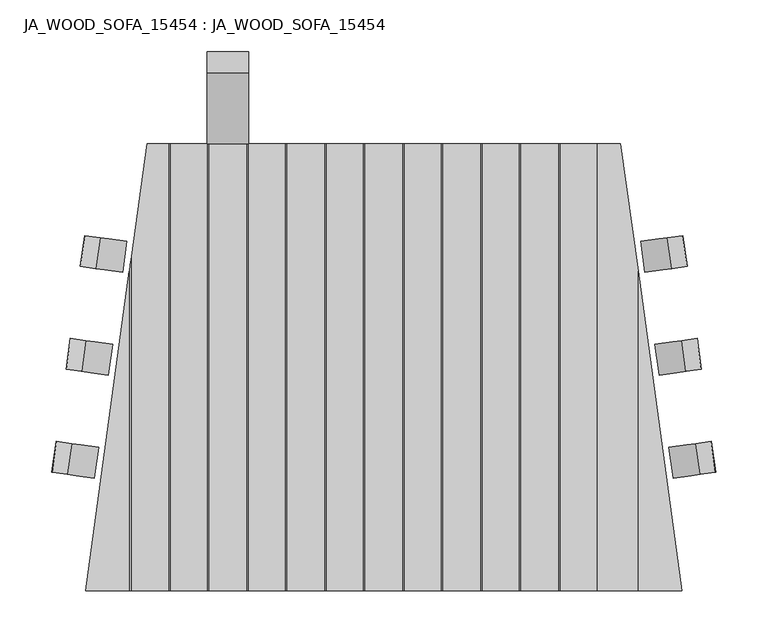
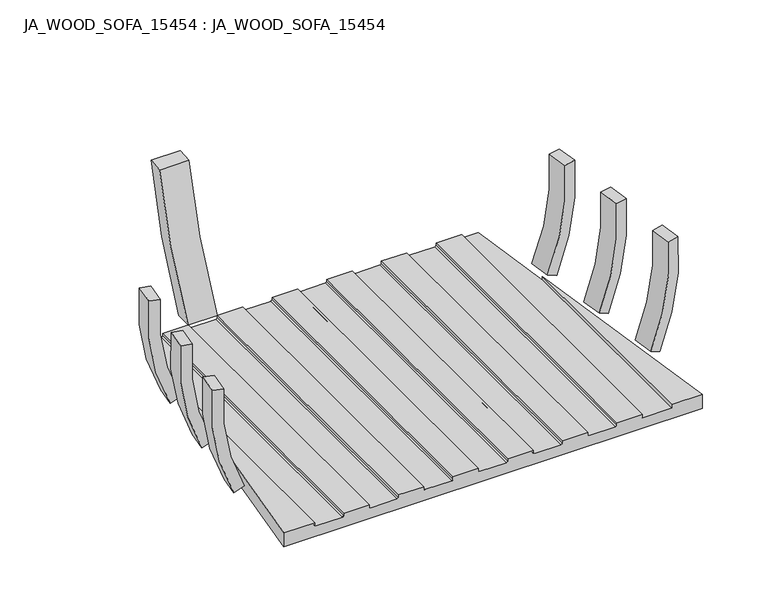
"""IFC4 building model written with IfcOpenShell, lengths in millimetres: furniture geometry, JA_WOOD_SOFA_15454 : JA_WOOD_SOFA_15454."""

from ifc_helpers import new_model, si_unit, point, frame, frame_2d, origin, origin_2d, place, context, project, spatial, polyline, circle_curve, ellipse_curve, trimmed, segment, composite_curve, outline, extrude, source, transform, mapped, element, save
from ifc_brep_helpers import plane_surface, revolved_surface, advanced_brep


def ja_wood_sofa_15454_ja_wood_sofa_15454_1d85e86b(model_context):
    return source(origin(), model_context, "Body", "SolidModel", [
        extrude(outline(composite_curve([segment(trimmed(circle_curve(frame_2d((-81.7276373, 616.3111076)), 600.0), [point((440.0, 320.0))], [point((507.7138581, 504.2453967))], True, "CARTESIAN"), True, "CONTINUOUS"), segment(polyline([(507.7138581, 504.2453967), (528.3899255, 506.0543182)]), True, "CONTINUOUS"), segment(trimmed(circle_curve(frame_2d((-81.7276373, 616.3111076)), 620.0), [point((528.3899255, 506.0543182))], [point((462.8820647, 320.0))], False, "CARTESIAN"), True, "CONTINUOUS"), segment(polyline([(462.8820647, 320.0), (440.0, 320.0)]), True, "CONTINUOUS")], self_intersect=False)), frame((-170.0, 0.0, 0.0), z_axis=(1.0, 0.0, 0.0), x_axis=(0.0, 1.0, 0.0)), (0.0, 0.0, 1.0), 40.0),
        extrude(outline(composite_curve([segment(trimmed(circle_curve(origin_2d(), 286.25), [point((246.9486899, -144.7598254))], [point((286.25, 0.0))], True, "CARTESIAN"), True, "CONTINUOUS"), segment(polyline([(286.25, 0.0), (301.2499999, -1e-07)]), True, "CONTINUOUS"), segment(trimmed(circle_curve(origin_2d(), 301.25), [point((301.2499999, -1e-07))], [point((259.8892326, -152.3454931))], False, "CARTESIAN"), True, "CONTINUOUS"), segment(polyline([(259.8892326, -152.3454931), (246.9486899, -144.7598254)]), True, "CONTINUOUS")], self_intersect=False)), frame((-22.2448942, 82.953428, 441.8308906), z_axis=(0.13632983976605592, 0.99066350230003, 0.0), x_axis=(-0.9866030973847555, 0.1357710684474402, 0.09044636644690265)), (0.0, 0.0, 1.0), 30.0),
        extrude(outline(composite_curve([segment(trimmed(circle_curve(origin_2d(), 286.25), [point((246.9486899, -144.7598254))], [point((286.25, 0.0))], True, "CARTESIAN"), True, "CONTINUOUS"), segment(polyline([(286.25, 0.0), (301.25, -1e-07)]), True, "CONTINUOUS"), segment(trimmed(circle_curve(origin_2d(), 301.25), [point((301.25, -1e-07))], [point((259.8892326, -152.3454931))], False, "CARTESIAN"), True, "CONTINUOUS"), segment(polyline([(259.8892326, -152.3454931), (246.9486899, -144.7598254)]), True, "CONTINUOUS")], self_intersect=False)), frame((-8.6188139, 182.0207281, 441.8308906), z_axis=(0.13632983976605592, 0.99066350230003, 0.0), x_axis=(-0.9866030973847555, 0.1357710684474402, 0.09044636644690265)), (0.0, 0.0, 1.0), 30.0),
        extrude(outline(composite_curve([segment(trimmed(circle_curve(origin_2d(), 286.25), [point((246.94869, -144.7598254))], [point((286.25, 0.0))], True, "CARTESIAN"), True, "CONTINUOUS"), segment(polyline([(286.25, 0.0), (301.25, -1e-07)]), True, "CONTINUOUS"), segment(trimmed(circle_curve(origin_2d(), 301.25), [point((301.25, -1e-07))], [point((259.8892326, -152.3454931))], False, "CARTESIAN"), True, "CONTINUOUS"), segment(polyline([(259.8892326, -152.3454931), (246.94869, -144.7598254)]), True, "CONTINUOUS")], self_intersect=False)), frame((5.0141701, 281.0870783, 441.8308906), z_axis=(0.13632983976605592, 0.99066350230003, 0.0), x_axis=(-0.9866030973847555, 0.1357710684474402, 0.09044636644690265)), (0.0, 0.0, 1.0), 30.0),
        extrude(outline(composite_curve([segment(trimmed(circle_curve(origin_2d(), 301.25), [point((259.8892326, 152.3454931))], [point((301.2499999, 1e-07))], False, "CARTESIAN"), True, "CONTINUOUS"), segment(polyline([(301.2499999, 1e-07), (286.25, 0.0)]), True, "CONTINUOUS"), segment(trimmed(circle_curve(origin_2d(), 286.25), [point((286.25, 0.0))], [point((246.9486899, 144.7598254))], True, "CARTESIAN"), True, "CONTINUOUS"), segment(polyline([(246.9486899, 144.7598254), (259.8892326, 152.3454931)]), True, "CONTINUOUS")], self_intersect=False)), frame((22.2448942, 82.953428, 441.8308906), z_axis=(-0.13632983976605592, 0.99066350230003, 0.0), x_axis=(0.9866030973847555, 0.1357710684474402, 0.09044636644690265)), (0.0, 0.0, 1.0), 30.0),
        extrude(outline(composite_curve([segment(trimmed(circle_curve(origin_2d(), 301.25), [point((259.8892326, 152.3454931))], [point((301.25, 1e-07))], False, "CARTESIAN"), True, "CONTINUOUS"), segment(polyline([(301.25, 1e-07), (286.25, 0.0)]), True, "CONTINUOUS"), segment(trimmed(circle_curve(origin_2d(), 286.25), [point((286.25, 0.0))], [point((246.9486899, 144.7598254))], True, "CARTESIAN"), True, "CONTINUOUS"), segment(polyline([(246.9486899, 144.7598254), (259.8892326, 152.3454931)]), True, "CONTINUOUS")], self_intersect=False)), frame((8.6188139, 182.0207281, 441.8308906), z_axis=(-0.13632983976605592, 0.99066350230003, 0.0), x_axis=(0.9866030973847555, 0.1357710684474402, 0.09044636644690265)), (0.0, 0.0, 1.0), 30.0),
        extrude(outline(composite_curve([segment(trimmed(circle_curve(origin_2d(), 301.25), [point((259.8892326, 152.3454931))], [point((301.25, 1e-07))], False, "CARTESIAN"), True, "CONTINUOUS"), segment(polyline([(301.25, 1e-07), (286.25, 0.0)]), True, "CONTINUOUS"), segment(trimmed(circle_curve(origin_2d(), 286.25), [point((286.25, 0.0))], [point((246.94869, 144.7598254))], True, "CARTESIAN"), True, "CONTINUOUS"), segment(polyline([(246.94869, 144.7598254), (259.8892326, 152.3454931)]), True, "CONTINUOUS")], self_intersect=False)), frame((-5.0141701, 281.0870783, 441.8308906), z_axis=(-0.13632983976605592, 0.99066350230003, 0.0), x_axis=(0.9866030973847555, 0.1357710684474402, 0.09044636644690265)), (0.0, 0.0, 1.0), 30.0),
        advanced_brep(
        [(-20.0, 10.0, 317.0), (-20.0, 440.0, 317.0), (-20.0, 440.0, 320.0), (-20.0, 10.0, 320.0), (18.0, 10.0, 315.0), (18.0, 440.0, 315.0), (-18.0, 440.0, 315.0), (-18.0, 10.0, 315.0), (20.0, 440.0, 317.0), (20.0, 10.0, 317.0), (20.0, 10.0, 320.0), (20.0, 440.0, 320.0), (55.0, 10.0, 317.0), (55.0, 440.0, 317.0), (55.0, 440.0, 320.0), (55.0, 10.0, 320.0), (93.0, 10.0, 315.0), (93.0, 440.0, 315.0), (57.0, 440.0, 315.0), (57.0, 10.0, 315.0), (95.0, 440.0, 317.0), (95.0, 10.0, 317.0), (95.0, 10.0, 320.0), (95.0, 440.0, 320.0), (130.0, 10.0, 317.0), (130.0, 440.0, 317.0), (130.0, 440.0, 320.0), (130.0, 10.0, 320.0), (168.0, 10.0, 315.0), (168.0, 440.0, 315.0), (132.0, 440.0, 315.0), (132.0, 10.0, 315.0), (170.0, 440.0, 317.0), (170.0, 10.0, 317.0), (170.0, 10.0, 320.0), (170.0, 440.0, 320.0), (-170.0, 10.0, 317.0), (-170.0, 440.0, 317.0), (-170.0, 440.0, 320.0), (-170.0, 10.0, 320.0), (-132.0, 10.0, 315.0), (-132.0, 440.0, 315.0), (-168.0, 440.0, 315.0), (-168.0, 10.0, 315.0), (-130.0, 440.0, 317.0), (-130.0, 10.0, 317.0), (-130.0, 10.0, 320.0), (-130.0, 440.0, 320.0), (-95.0, 10.0, 317.0), (-95.0, 440.0, 317.0), (-95.0, 440.0, 320.0), (-95.0, 10.0, 320.0), (-57.0, 10.0, 315.0), (-57.0, 440.0, 315.0), (-93.0, 440.0, 315.0), (-93.0, 10.0, 315.0), (-55.0, 440.0, 317.0), (-55.0, 10.0, 317.0), (-55.0, 10.0, 320.0), (-55.0, 440.0, 320.0), (-245.0, 10.0, 317.0), (-245.0, 317.1484871, 317.0), (-245.0, 317.1484871, 320.0), (-245.0, 10.0, 320.0), (-207.0, 10.0, 315.0), (-207.0, 440.0, 315.0), (-228.0938285, 440.0, 315.0), (-243.0, 331.6818204, 315.0), (-243.0, 10.0, 315.0), (-205.0, 440.0, 317.0), (-205.0, 10.0, 317.0), (-205.0, 10.0, 320.0), (-205.0, 440.0, 320.0), (205.0, 10.0, 315.0), (205.0, 440.0, 315.0), (205.0, 440.0, 320.0), (205.0, 10.0, 320.0), (245.0, 10.0, 315.0), (245.0, 317.1484871, 315.0), (228.0938285, 440.0, 315.0), (245.0, 10.0, 320.0), (245.0, 317.1484871, 320.0), (-287.2681404, 10.0, 320.0), (287.2681404, 10.0, 320.0), (-228.0938285, 440.0, 300.0), (228.0938285, 440.0, 300.0), (287.2681404, 10.0, 300.0), (-287.2681404, 10.0, 300.0)],
        [
            (0, 1),
            (1, 2),
            (2, 3),
            (3, 0),
            (4, 5),
            (5, 6),
            (6, 7),
            (7, 4),
            (8, 9),
            (9, 10),
            (10, 11),
            (11, 8),
            (12, 13),
            (13, 14),
            (14, 15),
            (15, 12),
            (16, 17),
            (17, 18),
            (18, 19),
            (19, 16),
            (20, 21),
            (21, 22),
            (22, 23),
            (23, 20),
            (24, 25),
            (25, 26),
            (26, 27),
            (27, 24),
            (28, 29),
            (29, 30),
            (30, 31),
            (31, 28),
            (32, 33),
            (33, 34),
            (34, 35),
            (35, 32),
            (36, 37),
            (37, 38),
            (38, 39),
            (39, 36),
            (40, 41),
            (41, 42),
            (42, 43),
            (43, 40),
            (44, 45),
            (45, 46),
            (46, 47),
            (47, 44),
            (48, 49),
            (49, 50),
            (50, 51),
            (51, 48),
            (52, 53),
            (53, 54),
            (54, 55),
            (55, 52),
            (56, 57),
            (57, 58),
            (58, 59),
            (59, 56),
            (60, 61),
            (61, 62),
            (62, 63),
            (63, 60),
            (64, 65),
            (65, 66),
            (66, 67),
            (67, 68),
            (68, 64),
            (69, 70),
            (70, 71),
            (71, 72),
            (72, 69),
            (73, 74),
            (74, 75),
            (75, 76),
            (76, 73),
            (73, 77),
            (77, 78),
            (78, 79),
            (79, 74),
            (77, 80),
            (80, 81),
            (81, 78),
            (62, 82),
            (82, 63),
            (10, 15),
            (14, 11),
            (22, 27),
            (26, 23),
            (46, 51),
            (50, 47),
            (58, 3),
            (2, 59),
            (71, 39),
            (38, 72),
            (34, 76),
            (75, 35),
            (80, 83),
            (83, 81),
            (84, 85),
            (85, 86),
            (86, 87),
            (87, 84),
            (87, 82),
            (61, 67, ellipse_curve(frame((-243.0, 331.6818204, 317.0), z_axis=(0.9906635023000295, -0.13632983976605914, 0.0), x_axis=(-0.13632983976605917, -0.9906635023000296, 0.0)), 14.6703026, 2.0)),
            (66, 84),
            (86, 83),
            (33, 28, circle_curve(frame((168.0, 10.0, 317.0), z_axis=(0.0, 1.0, 0.0), x_axis=(1.0, 0.0, 0.0)), 2.0)),
            (31, 24, circle_curve(frame((132.0, 10.0, 317.0), z_axis=(0.0, 1.0, 0.0), x_axis=(1.0, 0.0, 0.0)), 2.0)),
            (21, 16, circle_curve(frame((93.0, 10.0, 317.0), z_axis=(0.0, 1.0, 0.0), x_axis=(1.0, 0.0, 0.0)), 2.0)),
            (19, 12, circle_curve(frame((57.0, 10.0, 317.0), z_axis=(0.0, 1.0, 0.0), x_axis=(1.0, 0.0, 0.0)), 2.0)),
            (9, 4, circle_curve(frame((18.0, 10.0, 317.0), z_axis=(0.0, 1.0, 0.0), x_axis=(1.0, 0.0, 0.0)), 2.0)),
            (7, 0, circle_curve(frame((-18.0, 10.0, 317.0), z_axis=(0.0, 1.0, 0.0), x_axis=(1.0, 0.0, 0.0)), 2.0)),
            (57, 52, circle_curve(frame((-57.0, 10.0, 317.0), z_axis=(0.0, 1.0, 0.0), x_axis=(1.0, 0.0, 0.0)), 2.0)),
            (55, 48, circle_curve(frame((-93.0, 10.0, 317.0), z_axis=(0.0, 1.0, 0.0), x_axis=(1.0, 0.0, 0.0)), 2.0)),
            (45, 40, circle_curve(frame((-132.0, 10.0, 317.0), z_axis=(0.0, 1.0, 0.0), x_axis=(1.0, 0.0, 0.0)), 2.0)),
            (43, 36, circle_curve(frame((-168.0, 10.0, 317.0), z_axis=(0.0, 1.0, 0.0), x_axis=(1.0, 0.0, 0.0)), 2.0)),
            (70, 64, circle_curve(frame((-207.0, 10.0, 317.0), z_axis=(0.0, 1.0, 0.0), x_axis=(1.0, 0.0, 0.0)), 2.0)),
            (68, 60, circle_curve(frame((-243.0, 10.0, 317.0), z_axis=(0.0, 1.0, 0.0), x_axis=(1.0, 0.0, 0.0)), 2.0)),
            (85, 79),
            (65, 69, circle_curve(frame((-207.0, 440.0, 317.0), z_axis=(0.0, -1.0, 0.0), x_axis=(1.0, 0.0, 0.0)), 2.0)),
            (37, 42, circle_curve(frame((-168.0, 440.0, 317.0), z_axis=(0.0, -1.0, 0.0), x_axis=(1.0, 0.0, 0.0)), 2.0)),
            (41, 44, circle_curve(frame((-132.0, 440.0, 317.0), z_axis=(0.0, -1.0, 0.0), x_axis=(1.0, 0.0, 0.0)), 2.0)),
            (49, 54, circle_curve(frame((-93.0, 440.0, 317.0), z_axis=(0.0, -1.0, 0.0), x_axis=(1.0, 0.0, 0.0)), 2.0)),
            (53, 56, circle_curve(frame((-57.0, 440.0, 317.0), z_axis=(0.0, -1.0, 0.0), x_axis=(1.0, 0.0, 0.0)), 2.0)),
            (1, 6, circle_curve(frame((-18.0, 440.0, 317.0), z_axis=(0.0, -1.0, 0.0), x_axis=(1.0, 0.0, 0.0)), 2.0)),
            (5, 8, circle_curve(frame((18.0, 440.0, 317.0), z_axis=(0.0, -1.0, 0.0), x_axis=(1.0, 0.0, 0.0)), 2.0)),
            (13, 18, circle_curve(frame((57.0, 440.0, 317.0), z_axis=(0.0, -1.0, 0.0), x_axis=(1.0, 0.0, 0.0)), 2.0)),
            (17, 20, circle_curve(frame((93.0, 440.0, 317.0), z_axis=(0.0, -1.0, 0.0), x_axis=(1.0, 0.0, 0.0)), 2.0)),
            (25, 30, circle_curve(frame((132.0, 440.0, 317.0), z_axis=(0.0, -1.0, 0.0), x_axis=(1.0, 0.0, 0.0)), 2.0)),
            (29, 32, circle_curve(frame((168.0, 440.0, 317.0), z_axis=(0.0, -1.0, 0.0), x_axis=(1.0, 0.0, 0.0)), 2.0)),
        ],
        [
            plane_surface(frame((-20.0, 10.0, 320.0), z_axis=(1.0, 0.0, 0.0), x_axis=(0.0, 1.0, 0.0))),
            plane_surface(frame((-18.0, 10.0, 315.0), z_axis=(0.0, 0.0, 1.0), x_axis=(0.0, 1.0, 0.0))),
            plane_surface(frame((20.0, 10.0, 317.0), z_axis=(-1.0, 0.0, 0.0), x_axis=(0.0, 1.0, 0.0))),
            plane_surface(frame((55.0, 10.0, 320.0), z_axis=(1.0, 0.0, 0.0), x_axis=(0.0, 1.0, 0.0))),
            plane_surface(frame((57.0, 10.0, 315.0), z_axis=(0.0, 0.0, 1.0), x_axis=(0.0, 1.0, 0.0))),
            plane_surface(frame((95.0, 10.0, 317.0), z_axis=(-1.0, 0.0, 0.0), x_axis=(0.0, 1.0, 0.0))),
            plane_surface(frame((130.0, 10.0, 320.0), z_axis=(1.0, 0.0, 0.0), x_axis=(0.0, 1.0, 0.0))),
            plane_surface(frame((132.0, 10.0, 315.0), z_axis=(0.0, 0.0, 1.0), x_axis=(0.0, 1.0, 0.0))),
            plane_surface(frame((170.0, 10.0, 317.0), z_axis=(-1.0, 0.0, 0.0), x_axis=(0.0, 1.0, 0.0))),
            plane_surface(frame((-170.0, 10.0, 320.0), z_axis=(1.0, 0.0, 0.0), x_axis=(0.0, 1.0, 0.0))),
            plane_surface(frame((-168.0, 10.0, 315.0), z_axis=(0.0, 0.0, 1.0), x_axis=(0.0, 1.0, 0.0))),
            plane_surface(frame((-130.0, 10.0, 317.0), z_axis=(-1.0, 0.0, 0.0), x_axis=(0.0, 1.0, 0.0))),
            plane_surface(frame((-95.0, 10.0, 320.0), z_axis=(1.0, 0.0, 0.0), x_axis=(0.0, 1.0, 0.0))),
            plane_surface(frame((-93.0, 10.0, 315.0), z_axis=(0.0, 0.0, 1.0), x_axis=(0.0, 1.0, 0.0))),
            plane_surface(frame((-55.0, 10.0, 317.0), z_axis=(-1.0, 0.0, 0.0), x_axis=(0.0, 1.0, 0.0))),
            plane_surface(frame((-245.0, 10.0, 320.0), z_axis=(1.0, 0.0, 0.0), x_axis=(0.0, 1.0, 0.0))),
            plane_surface(frame((-243.0, 10.0, 315.0), z_axis=(0.0, 0.0, 1.0), x_axis=(0.0, 1.0, 0.0))),
            plane_surface(frame((-205.0, 10.0, 317.0), z_axis=(-1.0, 0.0, 0.0), x_axis=(0.0, 1.0, 0.0))),
            plane_surface(frame((205.0, 10.0, 320.0), z_axis=(1.0, 0.0, 0.0), x_axis=(0.0, 1.0, 0.0))),
            plane_surface(frame((205.0, 10.0, 315.0), z_axis=(0.0, 0.0, 1.0), x_axis=(0.0, 1.0, 0.0))),
            plane_surface(frame((245.0, 10.0, 315.0), z_axis=(-1.0, 0.0, 0.0), x_axis=(0.0, 1.0, 0.0))),
            plane_surface(frame((-287.6258394, 7.4007211, 320.0), z_axis=(0.0, 0.0, 1.0), x_axis=(-0.13632983976605914, -0.9906635023000295, 0.0))),
            plane_surface(frame((-287.6258394, 7.4007211, 300.0), z_axis=(0.0, 0.0, -1.0), x_axis=(0.13632983976605914, 0.9906635023000295, 0.0))),
            plane_surface(frame((-228.0938285, 440.0, 320.0), z_axis=(-0.9906635023000295, 0.13632983976605914, 0.0), x_axis=(0.0, 0.0, -1.0))),
            plane_surface(frame((-287.2681404, 10.0, 320.0), z_axis=(0.0, -1.0, 0.0), x_axis=(0.0, 0.0, -1.0))),
            plane_surface(frame((287.2681404, 10.0, 320.0), z_axis=(0.9906635023000295, 0.13632983976605914, 0.0), x_axis=(0.0, 0.0, -1.0))),
            plane_surface(frame((228.0938285, 440.0, 320.0), z_axis=(0.0, 1.0, 0.0), x_axis=(0.0, 0.0, -1.0))),
            revolved_surface(polyline([(-16.0, 10.0, 317.0), (-16.0, 440.0, 317.0)]), (-18.0, 440.0, 317.0), (0.0, -1.0, 0.0)),
            revolved_surface(polyline([(20.0, 10.0, 317.0), (20.0, 440.0, 317.0)]), (18.0, 440.0, 317.0), (0.0, -1.0, 0.0)),
            revolved_surface(polyline([(59.0, 10.0, 317.0), (59.0, 440.0, 317.0)]), (57.0, 440.0, 317.0), (0.0, -1.0, 0.0)),
            revolved_surface(polyline([(95.0, 10.0, 317.0), (95.0, 440.0, 317.0)]), (93.0, 440.0, 317.0), (0.0, -1.0, 0.0)),
            revolved_surface(polyline([(134.0, 10.0, 317.0), (134.0, 440.0, 317.0)]), (132.0, 440.0, 317.0), (0.0, -1.0, 0.0)),
            revolved_surface(polyline([(170.0, 10.0, 317.0), (170.0, 440.0, 317.0)]), (168.0, 440.0, 317.0), (0.0, -1.0, 0.0)),
            revolved_surface(polyline([(-166.0, 10.0, 317.0), (-166.0, 440.0, 317.0)]), (-168.0, 440.0, 317.0), (0.0, -1.0, 0.0)),
            revolved_surface(polyline([(-130.0, 10.0, 317.0), (-130.0, 440.0, 317.0)]), (-132.0, 440.0, 317.0), (0.0, -1.0, 0.0)),
            revolved_surface(polyline([(-91.0, 10.0, 317.0), (-91.0, 440.0, 317.0)]), (-93.0, 440.0, 317.0), (0.0, -1.0, 0.0)),
            revolved_surface(polyline([(-55.0, 10.0, 317.0), (-55.0, 440.0, 317.0)]), (-57.0, 440.0, 317.0), (0.0, -1.0, 0.0)),
            revolved_surface(polyline([(-241.0, 10.0, 317.0), (-241.0, 346.21515375351726, 317.0)]), (-243.0, 440.0, 317.0), (0.0, -1.0, 0.0)),
            revolved_surface(polyline([(-205.0, 10.0, 317.0), (-205.0, 440.0, 317.0)]), (-207.0, 440.0, 317.0), (0.0, -1.0, 0.0)),
        ],
        [
            (0, [[1, 2, 3, 4]]),
            (1, [[5, 6, 7, 8]]),
            (2, [[9, 10, 11, 12]]),
            (3, [[13, 14, 15, 16]]),
            (4, [[17, 18, 19, 20]]),
            (5, [[21, 22, 23, 24]]),
            (6, [[25, 26, 27, 28]]),
            (7, [[29, 30, 31, 32]]),
            (8, [[33, 34, 35, 36]]),
            (9, [[37, 38, 39, 40]]),
            (10, [[41, 42, 43, 44]]),
            (11, [[45, 46, 47, 48]]),
            (12, [[49, 50, 51, 52]]),
            (13, [[53, 54, 55, 56]]),
            (14, [[57, 58, 59, 60]]),
            (15, [[61, 62, 63, 64]]),
            (16, [[65, 66, 67, 68, 69]]),
            (17, [[70, 71, 72, 73]]),
            (18, [[74, 75, 76, 77]]),
            (19, [[-74, 78, 79, 80, 81]]),
            (20, [[-79, 82, 83, 84]]),
            (21, [[85, 86, -63]]),
            (21, [[87, -15, 88, -11]]),
            (21, [[89, -27, 90, -23]]),
            (21, [[91, -51, 92, -47]]),
            (21, [[93, -3, 94, -59]]),
            (21, [[95, -39, 96, -72]]),
            (21, [[97, -76, 98, -35]]),
            (21, [[99, 100, -83]]),
            (22, [[101, 102, 103, 104]]),
            (23, [[-104, 105, -85, -62, 106, -67, 107]]),
            (24, [[-103, 108, -99, -82, -78, -77, -97, -34, 109, -32, 110, -28, -89, -22, 111, -20, 112, -16, -87, -10, 113, -8, 114, -4, -93, -58, 115, -56, 116, -52, -91, -46, 117, -44, 118, -40, -95, -71, 119, -69, 120, -64, -86, -105]]),
            (25, [[-102, 121, -80, -84, -100, -108]]),
            (26, [[-101, -107, -66, 122, -73, -96, -38, 123, -42, 124, -48, -92, -50, 125, -54, 126, -60, -94, -2, 127, -6, 128, -12, -88, -14, 129, -18, 130, -24, -90, -26, 131, -30, 132, -36, -98, -75, -81, -121]]),
            (27, [[-1, -114, -7, -127]]),
            (28, [[-5, -113, -9, -128]]),
            (29, [[-13, -112, -19, -129]]),
            (30, [[-17, -111, -21, -130]]),
            (31, [[-25, -110, -31, -131]]),
            (32, [[-29, -109, -33, -132]]),
            (33, [[-37, -118, -43, -123]]),
            (34, [[-41, -117, -45, -124]]),
            (35, [[-49, -116, -55, -125]]),
            (36, [[-53, -115, -57, -126]]),
            (37, [[-68, -106, -61, -120]]),
            (38, [[-65, -119, -70, -122]]),
        ],
    ),
    ])


if __name__ == "__main__":
    model = new_model("IFC4")
    model_context = context("Model", 3, world=origin())
    ifc_project = project(units=[si_unit("LENGTHUNIT", "METRE", prefix="MILLI")], contexts=[model_context])
    site = spatial("IfcSite", under=ifc_project)
    building = spatial("IfcBuilding", under=site)
    placement = place(None, origin())
    ja_wood_sofa_15454_ja_wood_sofa_15454_shape = ja_wood_sofa_15454_ja_wood_sofa_15454_1d85e86b(model_context)
    element("IfcFurniture", 1, ObjectType="JA_WOOD_SOFA_15454 : JA_WOOD_SOFA_15454", at=placement, inside=building, context=model_context, shape_type="MappedRepresentation", body=[
        mapped(ja_wood_sofa_15454_ja_wood_sofa_15454_shape, transform((0.0, 0.0, 0.0), x_axis=(1.0, 0.0, 0.0), y_axis=(0.0, 1.0, 0.0), z_axis=(0.0, 0.0, 1.0))),
    ])
    save(model, "model.ifc")

# Revit data of these elements
# Type "JA_WOOD_SOFA_15454 : JA_WOOD_SOFA_15454"
#   LEG = WOOD FURNITURE - LEG
#   FRAME = WOOD FURNITURE - FRAME
#   Default Elevation = 0
# Element 1 (IfcFurniture, "JA_WOOD_SOFA_15454 : JA_WOOD_SOFA_15454")
#   Materials on its faces: "WOOD FURNITURE - LEG", "WOOD FURNITURE - FRAME"
# Materials
#   "WOOD FURNITURE - LEG": class "Generic", colour RGB 119 73 45, transparency 0, Cost = 0
#   "WOOD FURNITURE - FRAME": class "Generic", colour RGB 121 66 39, transparency 0, Cost = 0
